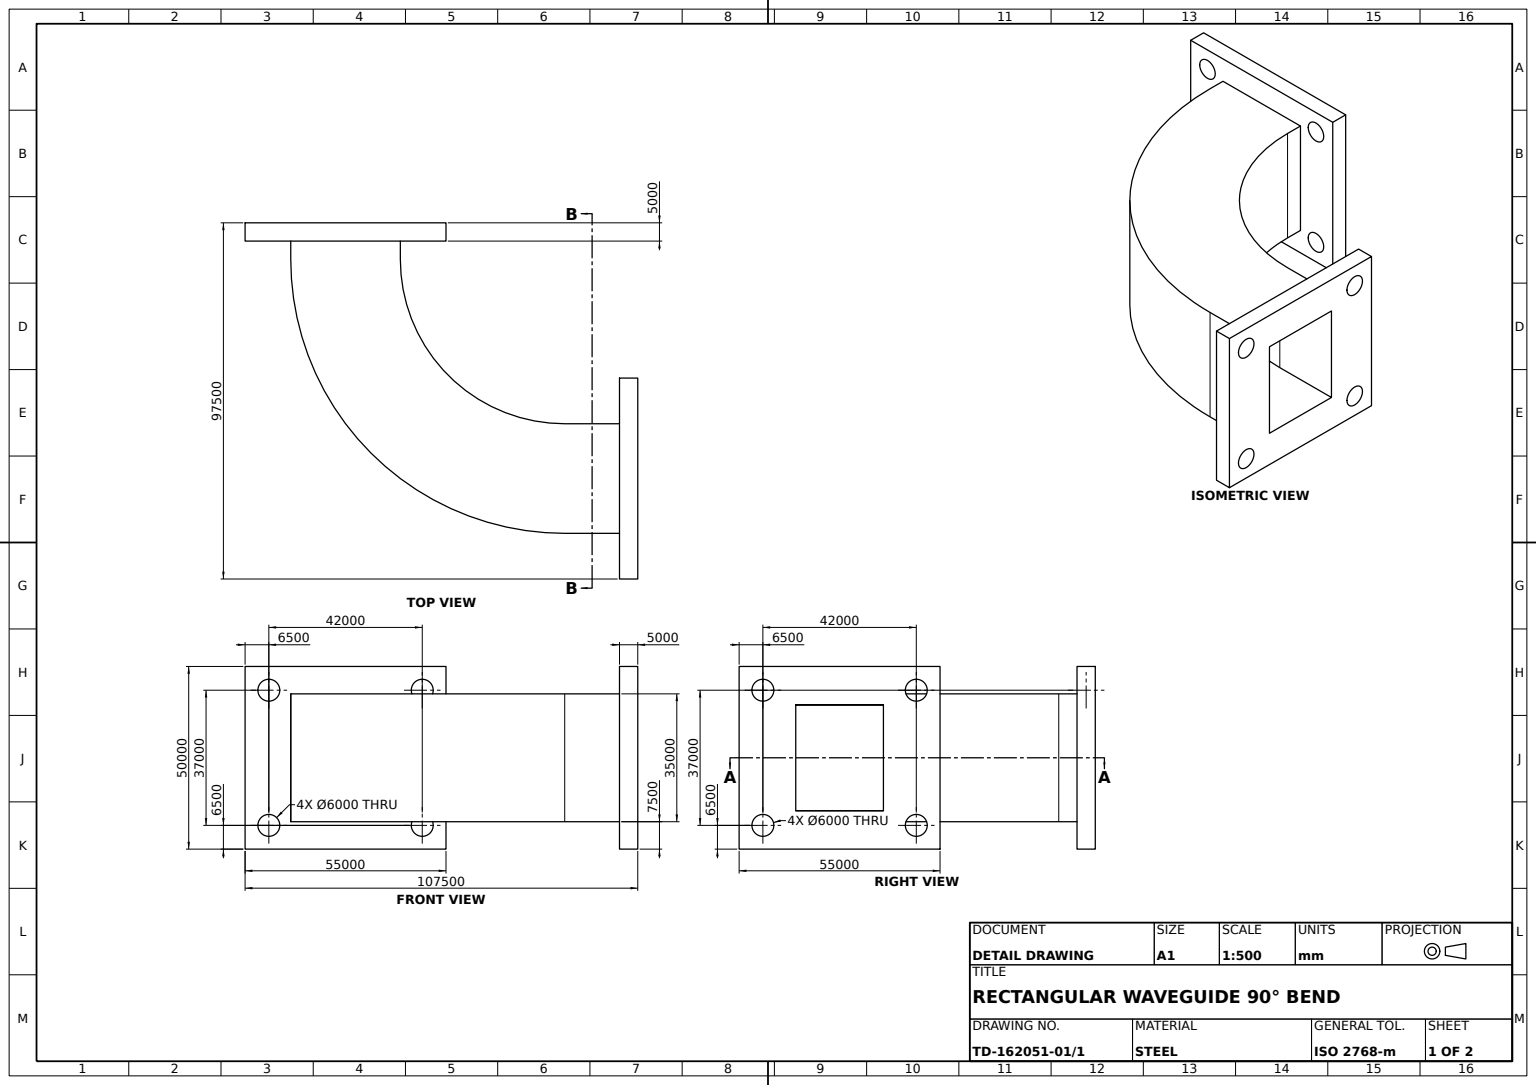
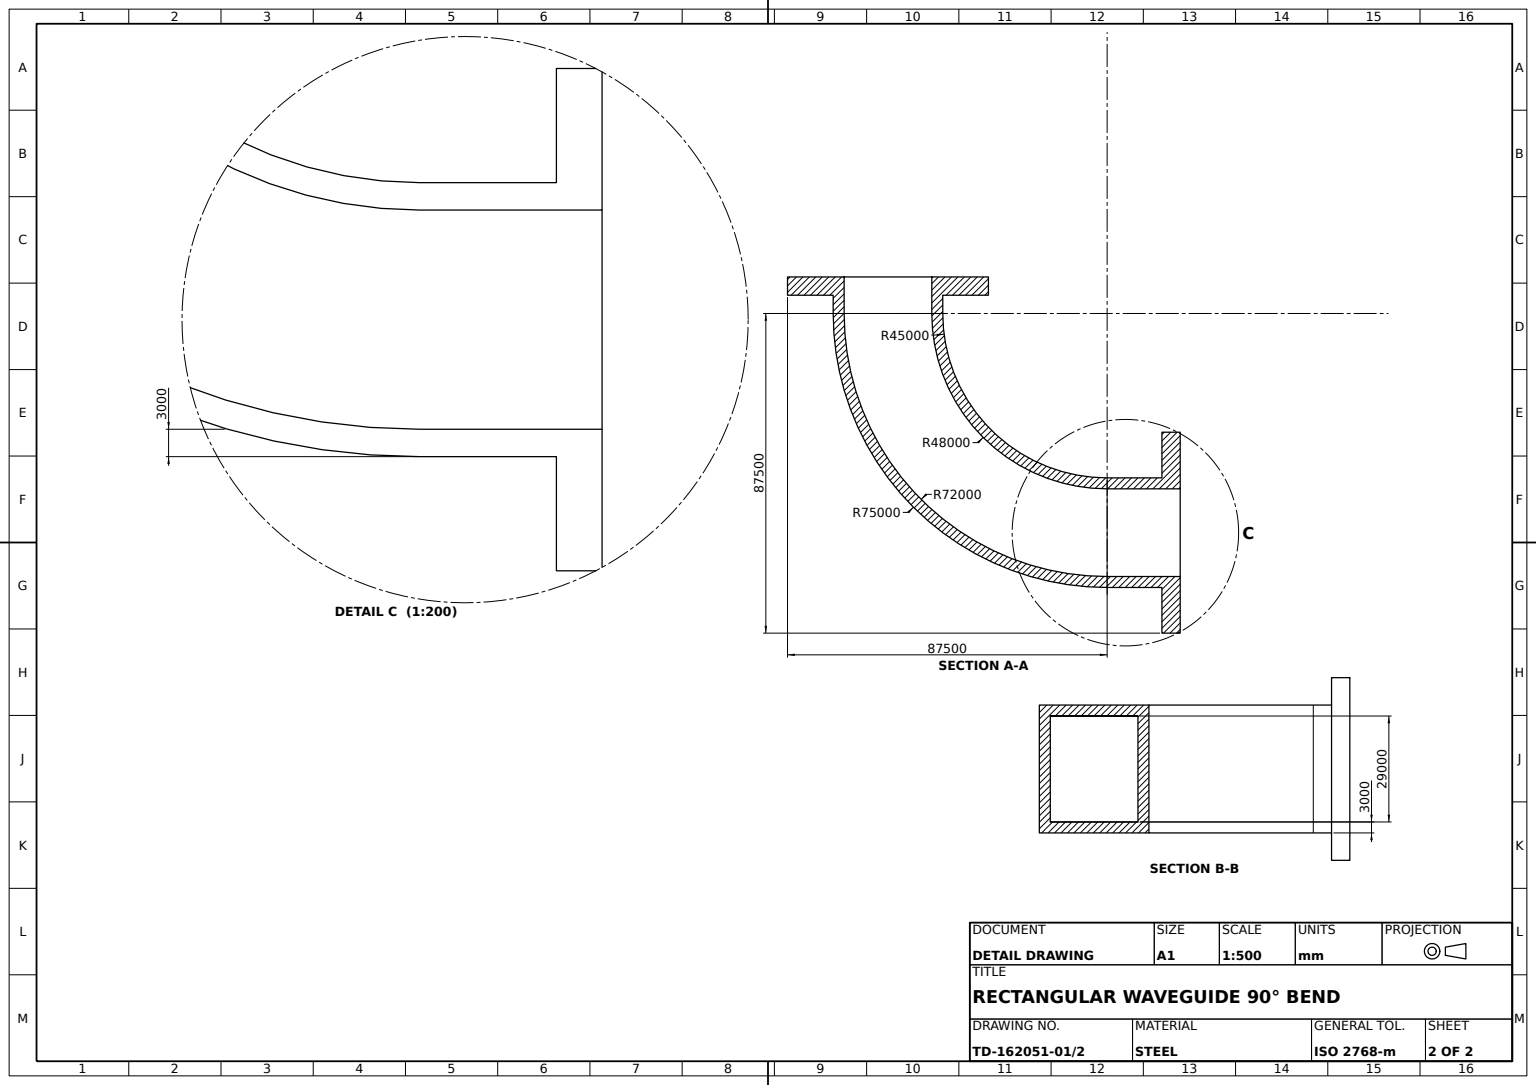
SolidWorks part; units mm, degrees
material "Plain Carbon Steel"
ref_plane "Front Plane" through (0, 0, 0) normal (0, 0, 1) x (1, 0, 0)
ref_plane "Top Plane" through (0, 0, 0) normal (0, 1, 0) x (1, 0, 0)
ref_plane "Right Plane" through (0, 0, 0) normal (1, 0, 0) x (0, 0, -1)
sketch "Duct Profile Sketch" plane through (0, 0, 0) normal (1, 0, 0) x (0, 0, -1)
  line L1 (-12000, 14500) -> (12000, 14500)
  line L2 (-12000, 14500) -> (-12000, -14500)
  line L3 (-12000, -14500) -> (12000, -14500)
  line L4 (12000, 14500) -> (12000, -14500)
  line L5 (-12000, 14500) -> (12000, -14500) construction
  line L6 (-12000, -14500) -> (12000, 14500) construction
  point P0 (0, 0)
  dimension "D1" = 24000
  dimension "D2" = 29000
sketch "Elbow Path Sketch" plane through (0, 0, 0) normal (0, 1, 0) x (1, 0, 0)
  line L0 (0, 0) -> (5000, 0)
  line L1 (65000, 60000) -> (65000, 75000)
  arc A0 (65000, 60000) -> (5000, 0) centre (5000, 60000) cw
  point P5 (65000, 0)
  dimension "D3" = 60000
  dimension "D1" = 75000
  dimension "D2" = 65000
sweep "Duct Elbow Thin Sweep" add profiles "Duct Profile Sketch" path "Elbow Path Sketch" parameters "D1"=3000
sketch "Flange A Sketch" plane through (0, 0, 0) normal (-1, 0, 0) x (0, 0, 1)
  line L1 (-27500, 25000) -> (27500, 25000)
  line L2 (-27500, 25000) -> (-27500, -25000)
  line L3 (-27500, -25000) -> (27500, -25000)
  line L4 (27500, 25000) -> (27500, -25000)
  line L5 (-27500, 25000) -> (27500, -25000) construction
  line L6 (-27500, -25000) -> (27500, 25000) construction
  line L7 (-12000, 14500) -> (12000, 14500)
  line L8 (-12000, 14500) -> (-12000, -14500)
  line L9 (-12000, -14500) -> (12000, -14500)
  line L10 (12000, 14500) -> (12000, -14500)
  line L11 (-12000, 14500) -> (12000, -14500) construction
  line L12 (-12000, -14500) -> (12000, 14500) construction
  point P0 (0, 0)
  point P6 (0, 0)
  dimension "D1" = 55000
  dimension "D2" = 50000
extrude "Flange A" add sketch "Flange A Sketch" along normal blind 5000
sketch "Flange B Sketch" plane through (0, 0, -75000) normal (0, 0, -1) x (-1, 0, 0)
  line L0 (0, 0) -> (-87772.7459, 0) construction
  line L1 (-65000, -14500) -> (-65000, 14500) construction
  line L2 (-77000, -14500) -> (-53000, -14500) construction
  line L3 (-53000, 14500) -> (-77000, 14500) construction
  line L5 (-92500, 25000) -> (-37500, 25000)
  line L6 (-92500, 25000) -> (-92500, -25000)
  line L7 (-92500, -25000) -> (-37500, -25000)
  line L8 (-37500, 25000) -> (-37500, -25000)
  line L9 (-92500, 25000) -> (-37500, -25000) construction
  line L10 (-92500, -25000) -> (-37500, 25000) construction
  line L11 (-77000, 14500) -> (-53000, 14500)
  line L12 (-77000, 14500) -> (-77000, -14500)
  line L13 (-77000, -14500) -> (-53000, -14500)
  line L14 (-53000, 14500) -> (-53000, -14500)
  line L15 (-77000, 14500) -> (-53000, -14500) construction
  line L16 (-77000, -14500) -> (-53000, 14500) construction
  point P9 (-65000, 0)
  point P14 (-65000, 0)
  dimension "D1" = 55000
  dimension "D2" = 50000
extrude "Flange B" add sketch "Flange B Sketch" along normal blind 5000
sketch "Flange B Bolt Holes Sketch" plane through (0, 0, -80000) normal (0, 0, -1) x (-1, 0, 0)
  line L0 (-92500, -25000) -> (-37500, -25000) construction
  line L1 (-92500, 25000) -> (-92500, -25000) construction
  line L2 (-37500, -25000) -> (-37500, 25000) construction
  line L3 (-37500, 25000) -> (-92500, 25000) construction
  circle A0 centre (-86000, 18500) radius 3000
  circle A1 centre (-44000, 18500) radius 3000
  circle A2 centre (-44000, -18500) radius 3000
  circle A3 centre (-86000, -18500) radius 3000
  dimension "D1" = 6000
  dimension "D2" = 6000
  dimension "D3" = 6000
  dimension "D4" = 6000
  dimension "D5" = 6500
  dimension "D6" = 6500
  dimension "D7" = 6500
  dimension "D8" = 6500
  dimension "D9" = 6500
  dimension "D10" = 6500
  dimension "D11" = 6500
  dimension "D12" = 6500
extrude "Flange B Bolt Holes 4x" cut sketch "Flange B Bolt Holes Sketch" against normal up to next
sketch "Flange A Bolt Holes Sketch" plane through (-5000, 0, 0) normal (-1, 0, 0) x (0, 0, 1)
  line L0 (27500, 25000) -> (-27500, 25000) construction
  line L1 (-27500, 25000) -> (-27500, -25000) construction
  line L2 (27500, -25000) -> (27500, 25000) construction
  line L3 (-27500, -25000) -> (27500, -25000) construction
  circle A0 centre (-21000, 18500) radius 3000
  circle A1 centre (21000, 18500) radius 3000
  circle A2 centre (21000, -18500) radius 3000
  circle A3 centre (-21000, -18500) radius 3000
  dimension "D1" = 6000
  dimension "D4" = 6000
  dimension "D7" = 6000
  dimension "D10" = 6000
  dimension "D2" = 6500
  dimension "D3" = 6500
  dimension "D5" = 6500
  dimension "D6" = 6500
  dimension "D8" = 6500
  dimension "D9" = 6500
  dimension "D11" = 6500
  dimension "D12" = 6500
extrude "Flange A Bolt Holes 4x" cut sketch "Flange A Bolt Holes Sketch" against normal up to next
